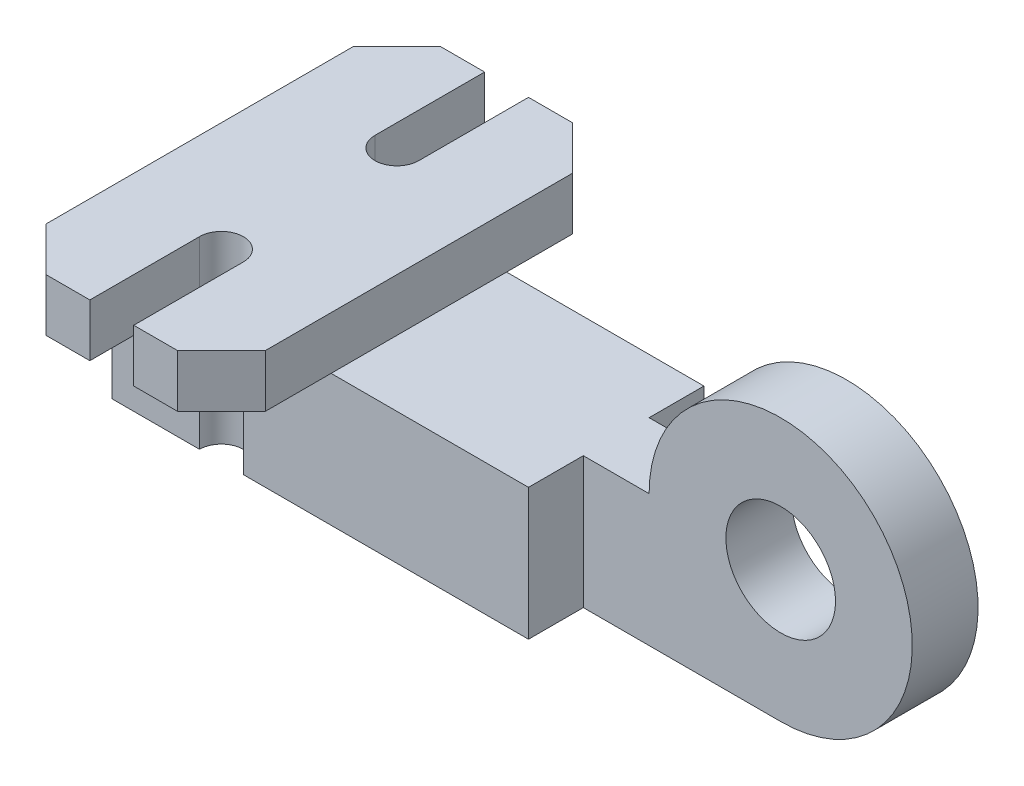
ISO-10303-21;
HEADER;
FILE_DESCRIPTION(('STEP AP214'),'2;1');
FILE_NAME('part.step','',(''),(''),'','','');
FILE_SCHEMA(('AUTOMOTIVE_DESIGN { 1 0 10303 214 1 1 1 1 }'));
ENDSEC;
DATA;
#1=APPLICATION_CONTEXT('core data for automotive mechanical design processes');
#2=APPLICATION_PROTOCOL_DEFINITION('international standard','automotive_design',2000,#1);
#3=PRODUCT_CONTEXT('',#1,'mechanical');
#4=PRODUCT('Part','Part','',(#3));
#5=PRODUCT_RELATED_PRODUCT_CATEGORY('part','',(#4));
#6=PRODUCT_DEFINITION_FORMATION('','',#4);
#7=PRODUCT_DEFINITION_CONTEXT('part definition',#1,'design');
#8=PRODUCT_DEFINITION('design','',#6,#7);
#9=PRODUCT_DEFINITION_SHAPE('','',#8);
#10=(LENGTH_UNIT() NAMED_UNIT(*) SI_UNIT(.MILLI.,.METRE.));
#11=(NAMED_UNIT(*) PLANE_ANGLE_UNIT() SI_UNIT($,.RADIAN.));
#12=(NAMED_UNIT(*) SI_UNIT($,.STERADIAN.) SOLID_ANGLE_UNIT());
#13=UNCERTAINTY_MEASURE_WITH_UNIT(LENGTH_MEASURE(1.E-05),#10,'distance_accuracy_value','');
#14=(GEOMETRIC_REPRESENTATION_CONTEXT(3) GLOBAL_UNCERTAINTY_ASSIGNED_CONTEXT((#13)) GLOBAL_UNIT_ASSIGNED_CONTEXT((#10,
#11,#12)) REPRESENTATION_CONTEXT('',''));
#15=CARTESIAN_POINT('',(0.,0.,0.));
#16=DIRECTION('',(0.,0.,1.));
#17=DIRECTION('',(1.,0.,0.));
#18=AXIS2_PLACEMENT_3D('',#15,#16,#17);
#19=CARTESIAN_POINT('',(0.,0.,20.));
#20=DIRECTION('',(0.,0.,-1.));
#21=DIRECTION('',(-1.,0.,0.));
#22=AXIS2_PLACEMENT_3D('',#19,#20,#21);
#23=PLANE('',#22);
#24=DIRECTION('',(-1.,0.,0.));
#25=VECTOR('',#24,1.);
#26=CARTESIAN_POINT('',(-47.5,15.,20.));
#27=LINE('',#26,#25);
#28=CARTESIAN_POINT('',(2.5,15.,20.));
#29=VERTEX_POINT('',#28);
#30=CARTESIAN_POINT('',(-17.5,15.,20.));
#31=VERTEX_POINT('',#30);
#32=EDGE_CURVE('E343',#29,#31,#27,.T.);
#33=ORIENTED_EDGE('',*,*,#32,.T.);
#34=DIRECTION('',(0.,1.,0.));
#35=VECTOR('',#34,1.);
#36=CARTESIAN_POINT('',(-17.5,-15.,20.));
#37=LINE('',#36,#35);
#38=CARTESIAN_POINT('',(-17.5,-15.,20.));
#39=VERTEX_POINT('',#38);
#40=EDGE_CURVE('E783',#39,#31,#37,.T.);
#41=ORIENTED_EDGE('',*,*,#40,.F.);
#42=DIRECTION('',(1.,0.,0.));
#43=VECTOR('',#42,1.);
#44=CARTESIAN_POINT('',(-47.5,-15.,20.));
#45=LINE('',#44,#43);
#46=CARTESIAN_POINT('',(47.5,-15.,20.));
#47=VERTEX_POINT('',#46);
#48=EDGE_CURVE('E347',#39,#47,#45,.T.);
#49=ORIENTED_EDGE('',*,*,#48,.T.);
#50=DIRECTION('',(0.,1.,0.));
#51=VECTOR('',#50,1.);
#52=CARTESIAN_POINT('',(47.5,-15.,20.));
#53=LINE('',#52,#51);
#54=CARTESIAN_POINT('',(47.5,15.,20.));
#55=VERTEX_POINT('',#54);
#56=EDGE_CURVE('E259',#47,#55,#53,.T.);
#57=ORIENTED_EDGE('',*,*,#56,.T.);
#58=EDGE_CURVE('E337',#55,#29,#27,.T.);
#59=ORIENTED_EDGE('',*,*,#58,.T.);
#60=EDGE_LOOP('',(#33,#41,#49,#57,#59));
#61=FACE_BOUND('',#60,.T.);
#62=ADVANCED_FACE('F50',(#61),#23,.F.);
#63=CARTESIAN_POINT('',(0.,0.,-20.));
#64=DIRECTION('',(0.,0.,-1.));
#65=DIRECTION('',(-1.,0.,0.));
#66=AXIS2_PLACEMENT_3D('',#63,#64,#65);
#67=PLANE('',#66);
#68=DIRECTION('',(0.,1.,0.));
#69=VECTOR('',#68,1.);
#70=CARTESIAN_POINT('',(-27.5,-15.,-20.));
#71=LINE('',#70,#69);
#72=CARTESIAN_POINT('',(-27.5,-15.,-20.));
#73=VERTEX_POINT('',#72);
#74=CARTESIAN_POINT('',(-27.5,15.,-20.));
#75=VERTEX_POINT('',#74);
#76=EDGE_CURVE('E792',#73,#75,#71,.T.);
#77=ORIENTED_EDGE('',*,*,#76,.F.);
#78=DIRECTION('',(1.,0.,0.));
#79=VECTOR('',#78,1.);
#80=CARTESIAN_POINT('',(-47.5,-15.,-20.));
#81=LINE('',#80,#79);
#82=CARTESIAN_POINT('',(-47.5,-15.,-20.));
#83=VERTEX_POINT('',#82);
#84=EDGE_CURVE('E248',#83,#73,#81,.T.);
#85=ORIENTED_EDGE('',*,*,#84,.F.);
#86=DIRECTION('',(0.,-1.,0.));
#87=VECTOR('',#86,1.);
#88=CARTESIAN_POINT('',(-47.5,-15.,-20.));
#89=LINE('',#88,#87);
#90=CARTESIAN_POINT('',(-47.5,15.,-20.));
#91=VERTEX_POINT('',#90);
#92=EDGE_CURVE('E260',#91,#83,#89,.T.);
#93=ORIENTED_EDGE('',*,*,#92,.F.);
#94=DIRECTION('',(-1.,0.,0.));
#95=VECTOR('',#94,1.);
#96=CARTESIAN_POINT('',(-47.5,15.,-20.));
#97=LINE('',#96,#95);
#98=EDGE_CURVE('E348',#75,#91,#97,.T.);
#99=ORIENTED_EDGE('',*,*,#98,.F.);
#100=EDGE_LOOP('',(#77,#85,#93,#99));
#101=FACE_BOUND('',#100,.T.);
#102=ADVANCED_FACE('F364',(#101),#67,.T.);
#103=CARTESIAN_POINT('',(0.,15.,0.));
#104=DIRECTION('',(0.,1.,0.));
#105=DIRECTION('',(0.,0.,1.));
#106=AXIS2_PLACEMENT_3D('',#103,#104,#105);
#107=PLANE('',#106);
#108=DIRECTION('',(0.,0.,1.));
#109=VECTOR('',#108,1.);
#110=CARTESIAN_POINT('',(-47.5,15.,-45.));
#111=LINE('',#110,#109);
#112=CARTESIAN_POINT('',(-47.5,15.,-35.));
#113=VERTEX_POINT('',#112);
#114=EDGE_CURVE('E328',#113,#91,#111,.T.);
#115=ORIENTED_EDGE('',*,*,#114,.F.);
#116=DIRECTION('',(-0.707106781186548,0.,0.707106781186547));
#117=VECTOR('',#116,1.);
#118=CARTESIAN_POINT('',(-47.5,15.,-35.));
#119=LINE('',#118,#117);
#120=CARTESIAN_POINT('',(-37.5,15.,-45.));
#121=VERTEX_POINT('',#120);
#122=EDGE_CURVE('E305',#113,#121,#119,.F.);
#123=ORIENTED_EDGE('',*,*,#122,.T.);
#124=DIRECTION('',(-1.,0.,0.));
#125=VECTOR('',#124,1.);
#126=CARTESIAN_POINT('',(-47.5,15.,-45.));
#127=LINE('',#126,#125);
#128=CARTESIAN_POINT('',(-27.5,15.,-45.));
#129=VERTEX_POINT('',#128);
#130=EDGE_CURVE('E334',#129,#121,#127,.T.);
#131=ORIENTED_EDGE('',*,*,#130,.F.);
#132=DIRECTION('',(0.,0.,1.));
#133=VECTOR('',#132,1.);
#134=CARTESIAN_POINT('',(-27.5,15.,0.));
#135=LINE('',#134,#133);
#136=EDGE_CURVE('E361',#129,#75,#135,.T.);
#137=ORIENTED_EDGE('',*,*,#136,.T.);
#138=ORIENTED_EDGE('',*,*,#98,.T.);
#139=EDGE_LOOP('',(#115,#123,#131,#137,#138));
#140=FACE_BOUND('',#139,.T.);
#141=ADVANCED_FACE('F363',(#140),#107,.F.);
#142=CARTESIAN_POINT('',(-47.5,27.,45.));
#143=DIRECTION('',(0.,0.,-1.));
#144=DIRECTION('',(-1.,0.,0.));
#145=AXIS2_PLACEMENT_3D('',#142,#143,#144);
#146=PLANE('',#145);
#147=DIRECTION('',(1.,0.,0.));
#148=VECTOR('',#147,1.);
#149=CARTESIAN_POINT('',(-47.5,15.,45.));
#150=LINE('',#149,#148);
#151=CARTESIAN_POINT('',(-17.5,15.,45.));
#152=VERTEX_POINT('',#151);
#153=CARTESIAN_POINT('',(-7.50000000000003,15.,45.));
#154=VERTEX_POINT('',#153);
#155=EDGE_CURVE('E322',#152,#154,#150,.T.);
#156=ORIENTED_EDGE('',*,*,#155,.T.);
#157=DIRECTION('',(0.,1.,0.));
#158=VECTOR('',#157,1.);
#159=CARTESIAN_POINT('',(-7.50000000000003,27.,45.));
#160=LINE('',#159,#158);
#161=CARTESIAN_POINT('',(-7.50000000000003,27.,45.));
#162=VERTEX_POINT('',#161);
#163=EDGE_CURVE('E306',#154,#162,#160,.T.);
#164=ORIENTED_EDGE('',*,*,#163,.T.);
#165=DIRECTION('',(1.,0.,0.));
#166=VECTOR('',#165,1.);
#167=CARTESIAN_POINT('',(-47.5,27.,45.));
#168=LINE('',#167,#166);
#169=CARTESIAN_POINT('',(-17.5,27.,45.));
#170=VERTEX_POINT('',#169);
#171=EDGE_CURVE('E392',#170,#162,#168,.T.);
#172=ORIENTED_EDGE('',*,*,#171,.F.);
#173=DIRECTION('',(0.,1.,0.));
#174=VECTOR('',#173,1.);
#175=CARTESIAN_POINT('',(-17.5,-15.,45.));
#176=LINE('',#175,#174);
#177=EDGE_CURVE('E789',#152,#170,#176,.T.);
#178=ORIENTED_EDGE('',*,*,#177,.F.);
#179=EDGE_LOOP('',(#156,#164,#172,#178));
#180=FACE_BOUND('',#179,.T.);
#181=ADVANCED_FACE('F567',(#180),#146,.F.);
#182=CARTESIAN_POINT('',(-47.5,27.,-45.));
#183=DIRECTION('',(0.,0.,1.));
#184=DIRECTION('',(1.,0.,0.));
#185=AXIS2_PLACEMENT_3D('',#182,#183,#184);
#186=PLANE('',#185);
#187=ORIENTED_EDGE('',*,*,#130,.T.);
#188=DIRECTION('',(0.,1.,0.));
#189=VECTOR('',#188,1.);
#190=CARTESIAN_POINT('',(-37.5,27.,-45.));
#191=LINE('',#190,#189);
#192=CARTESIAN_POINT('',(-37.5,27.,-45.));
#193=VERTEX_POINT('',#192);
#194=EDGE_CURVE('E302',#121,#193,#191,.T.);
#195=ORIENTED_EDGE('',*,*,#194,.T.);
#196=DIRECTION('',(-1.,0.,0.));
#197=VECTOR('',#196,1.);
#198=CARTESIAN_POINT('',(-47.5,27.,-45.));
#199=LINE('',#198,#197);
#200=CARTESIAN_POINT('',(-27.5,27.,-45.));
#201=VERTEX_POINT('',#200);
#202=EDGE_CURVE('E398',#201,#193,#199,.T.);
#203=ORIENTED_EDGE('',*,*,#202,.F.);
#204=DIRECTION('',(0.,1.,0.));
#205=VECTOR('',#204,1.);
#206=CARTESIAN_POINT('',(-27.5,-15.,-45.));
#207=LINE('',#206,#205);
#208=EDGE_CURVE('E770',#129,#201,#207,.T.);
#209=ORIENTED_EDGE('',*,*,#208,.F.);
#210=EDGE_LOOP('',(#187,#195,#203,#209));
#211=FACE_BOUND('',#210,.T.);
#212=ADVANCED_FACE('F579',(#211),#186,.F.);
#213=DIRECTION('',(0.,0.,-1.));
#214=VECTOR('',#213,1.);
#215=CARTESIAN_POINT('',(2.49999999999999,15.,-45.));
#216=LINE('',#215,#214);
#217=CARTESIAN_POINT('',(2.5,15.,35.));
#218=VERTEX_POINT('',#217);
#219=EDGE_CURVE('E330',#218,#29,#216,.T.);
#220=ORIENTED_EDGE('',*,*,#219,.F.);
#221=DIRECTION('',(0.707106781186548,0.,-0.707106781186547));
#222=VECTOR('',#221,1.);
#223=CARTESIAN_POINT('',(2.5,15.,35.));
#224=LINE('',#223,#222);
#225=EDGE_CURVE('E68',#218,#154,#224,.F.);
#226=ORIENTED_EDGE('',*,*,#225,.T.);
#227=ORIENTED_EDGE('',*,*,#155,.F.);
#228=DIRECTION('',(0.,0.,-1.));
#229=VECTOR('',#228,1.);
#230=CARTESIAN_POINT('',(-17.5,15.,0.));
#231=LINE('',#230,#229);
#232=EDGE_CURVE('E280',#152,#31,#231,.T.);
#233=ORIENTED_EDGE('',*,*,#232,.T.);
#234=ORIENTED_EDGE('',*,*,#32,.F.);
#235=EDGE_LOOP('',(#220,#226,#227,#233,#234));
#236=FACE_BOUND('',#235,.T.);
#237=ADVANCED_FACE('F566',(#236),#107,.F.);
#238=CARTESIAN_POINT('',(47.5,-15.,20.));
#239=DIRECTION('',(-1.,0.,0.));
#240=DIRECTION('',(0.,0.,1.));
#241=AXIS2_PLACEMENT_3D('',#238,#239,#240);
#242=PLANE('',#241);
#243=DIRECTION('',(0.,-1.,0.));
#244=VECTOR('',#243,1.);
#245=CARTESIAN_POINT('',(47.5,-15.,7.5));
#246=LINE('',#245,#244);
#247=CARTESIAN_POINT('',(47.5,15.,7.5));
#248=VERTEX_POINT('',#247);
#249=CARTESIAN_POINT('',(47.5,-15.,7.5));
#250=VERTEX_POINT('',#249);
#251=EDGE_CURVE('E810',#248,#250,#246,.T.);
#252=ORIENTED_EDGE('',*,*,#251,.F.);
#253=DIRECTION('',(0.,0.,-1.));
#254=VECTOR('',#253,1.);
#255=CARTESIAN_POINT('',(47.5,15.,20.));
#256=LINE('',#255,#254);
#257=EDGE_CURVE('E269',#55,#248,#256,.T.);
#258=ORIENTED_EDGE('',*,*,#257,.F.);
#259=ORIENTED_EDGE('',*,*,#56,.F.);
#260=DIRECTION('',(0.,0.,-1.));
#261=VECTOR('',#260,1.);
#262=CARTESIAN_POINT('',(47.5,-15.,20.));
#263=LINE('',#262,#261);
#264=EDGE_CURVE('E262',#47,#250,#263,.T.);
#265=ORIENTED_EDGE('',*,*,#264,.T.);
#266=EDGE_LOOP('',(#252,#258,#259,#265));
#267=FACE_BOUND('',#266,.T.);
#268=ADVANCED_FACE('F449',(#267),#242,.F.);
#269=CARTESIAN_POINT('',(-47.5,15.,20.));
#270=DIRECTION('',(0.,-1.,0.));
#271=DIRECTION('',(0.,0.,-1.));
#272=AXIS2_PLACEMENT_3D('',#269,#270,#271);
#273=PLANE('',#272);
#274=CARTESIAN_POINT('',(2.49999999999999,15.,-20.));
#275=VERTEX_POINT('',#274);
#276=EDGE_CURVE('E272',#29,#275,#216,.T.);
#277=ORIENTED_EDGE('',*,*,#276,.F.);
#278=ORIENTED_EDGE('',*,*,#58,.F.);
#279=ORIENTED_EDGE('',*,*,#257,.T.);
#280=DIRECTION('',(-1.,0.,0.));
#281=VECTOR('',#280,1.);
#282=CARTESIAN_POINT('',(47.5,15.,7.5));
#283=LINE('',#282,#281);
#284=CARTESIAN_POINT('',(62.5,15.,7.5));
#285=VERTEX_POINT('',#284);
#286=EDGE_CURVE('E805',#285,#248,#283,.T.);
#287=ORIENTED_EDGE('',*,*,#286,.F.);
#288=DIRECTION('',(0.,0.,-1.));
#289=VECTOR('',#288,1.);
#290=CARTESIAN_POINT('',(62.5,15.,7.5));
#291=LINE('',#290,#289);
#292=CARTESIAN_POINT('',(62.5,15.,-7.5));
#293=VERTEX_POINT('',#292);
#294=EDGE_CURVE('E385',#285,#293,#291,.T.);
#295=ORIENTED_EDGE('',*,*,#294,.T.);
#296=DIRECTION('',(-1.,0.,0.));
#297=VECTOR('',#296,1.);
#298=CARTESIAN_POINT('',(47.5,15.,-7.5));
#299=LINE('',#298,#297);
#300=CARTESIAN_POINT('',(47.5,15.,-7.5));
#301=VERTEX_POINT('',#300);
#302=EDGE_CURVE('E803',#293,#301,#299,.T.);
#303=ORIENTED_EDGE('',*,*,#302,.T.);
#304=CARTESIAN_POINT('',(47.5,15.,-20.));
#305=VERTEX_POINT('',#304);
#306=EDGE_CURVE('E267',#301,#305,#256,.T.);
#307=ORIENTED_EDGE('',*,*,#306,.T.);
#308=EDGE_CURVE('E257',#305,#275,#97,.T.);
#309=ORIENTED_EDGE('',*,*,#308,.T.);
#310=EDGE_LOOP('',(#277,#278,#279,#287,#295,#303,#307,#309));
#311=FACE_BOUND('',#310,.T.);
#312=ADVANCED_FACE('F448',(#311),#273,.F.);
#313=ORIENTED_EDGE('',*,*,#306,.F.);
#314=DIRECTION('',(0.,-1.,0.));
#315=VECTOR('',#314,1.);
#316=CARTESIAN_POINT('',(47.5,-15.,-7.5));
#317=LINE('',#316,#315);
#318=CARTESIAN_POINT('',(47.5,-15.,-7.5));
#319=VERTEX_POINT('',#318);
#320=EDGE_CURVE('E816',#301,#319,#317,.T.);
#321=ORIENTED_EDGE('',*,*,#320,.T.);
#322=CARTESIAN_POINT('',(47.5,-15.,-20.));
#323=VERTEX_POINT('',#322);
#324=EDGE_CURVE('E270',#319,#323,#263,.T.);
#325=ORIENTED_EDGE('',*,*,#324,.T.);
#326=DIRECTION('',(0.,1.,0.));
#327=VECTOR('',#326,1.);
#328=CARTESIAN_POINT('',(47.5,-15.,-20.));
#329=LINE('',#328,#327);
#330=EDGE_CURVE('E258',#323,#305,#329,.T.);
#331=ORIENTED_EDGE('',*,*,#330,.T.);
#332=EDGE_LOOP('',(#313,#321,#325,#331));
#333=FACE_BOUND('',#332,.T.);
#334=ADVANCED_FACE('F444',(#333),#242,.F.);
#335=CARTESIAN_POINT('',(-47.5,-15.,20.));
#336=DIRECTION('',(1.,0.,0.));
#337=DIRECTION('',(0.,0.,-1.));
#338=AXIS2_PLACEMENT_3D('',#335,#336,#337);
#339=PLANE('',#338);
#340=DIRECTION('',(0.,0.,1.));
#341=VECTOR('',#340,1.);
#342=CARTESIAN_POINT('',(-47.5,27.,-45.));
#343=LINE('',#342,#341);
#344=CARTESIAN_POINT('',(-47.5,27.,-35.));
#345=VERTEX_POINT('',#344);
#346=CARTESIAN_POINT('',(-47.5,27.,35.));
#347=VERTEX_POINT('',#346);
#348=EDGE_CURVE('E338',#345,#347,#343,.T.);
#349=ORIENTED_EDGE('',*,*,#348,.F.);
#350=DIRECTION('',(0.,-1.,0.));
#351=VECTOR('',#350,1.);
#352=CARTESIAN_POINT('',(-47.5,-15.,-35.));
#353=LINE('',#352,#351);
#354=EDGE_CURVE('E297',#345,#113,#353,.T.);
#355=ORIENTED_EDGE('',*,*,#354,.T.);
#356=ORIENTED_EDGE('',*,*,#114,.T.);
#357=ORIENTED_EDGE('',*,*,#92,.T.);
#358=DIRECTION('',(0.,0.,-1.));
#359=VECTOR('',#358,1.);
#360=CARTESIAN_POINT('',(-47.5,-15.,20.));
#361=LINE('',#360,#359);
#362=CARTESIAN_POINT('',(-47.5,-15.,20.));
#363=VERTEX_POINT('',#362);
#364=EDGE_CURVE('E266',#363,#83,#361,.T.);
#365=ORIENTED_EDGE('',*,*,#364,.F.);
#366=DIRECTION('',(0.,-1.,0.));
#367=VECTOR('',#366,1.);
#368=CARTESIAN_POINT('',(-47.5,-15.,20.));
#369=LINE('',#368,#367);
#370=CARTESIAN_POINT('',(-47.5,15.,20.));
#371=VERTEX_POINT('',#370);
#372=EDGE_CURVE('E345',#371,#363,#369,.T.);
#373=ORIENTED_EDGE('',*,*,#372,.F.);
#374=CARTESIAN_POINT('',(-47.5,15.,35.));
#375=VERTEX_POINT('',#374);
#376=EDGE_CURVE('E377',#371,#375,#111,.T.);
#377=ORIENTED_EDGE('',*,*,#376,.T.);
#378=DIRECTION('',(0.,1.,0.));
#379=VECTOR('',#378,1.);
#380=CARTESIAN_POINT('',(-47.5,-15.,35.));
#381=LINE('',#380,#379);
#382=EDGE_CURVE('E296',#375,#347,#381,.T.);
#383=ORIENTED_EDGE('',*,*,#382,.T.);
#384=EDGE_LOOP('',(#349,#355,#356,#357,#365,#373,#377,#383));
#385=FACE_BOUND('',#384,.T.);
#386=ADVANCED_FACE('F369',(#385),#339,.F.);
#387=CARTESIAN_POINT('',(-47.5,-15.,20.));
#388=DIRECTION('',(0.,1.,0.));
#389=DIRECTION('',(0.,0.,1.));
#390=AXIS2_PLACEMENT_3D('',#387,#388,#389);
#391=PLANE('',#390);
#392=ORIENTED_EDGE('',*,*,#84,.T.);
#393=CARTESIAN_POINT('',(-22.5,-15.,-20.));
#394=DIRECTION('',(0.,1.,0.));
#395=DIRECTION('',(0.,0.,1.));
#396=AXIS2_PLACEMENT_3D('',#393,#394,#395);
#397=CIRCLE('',#396,5.);
#398=CARTESIAN_POINT('',(-17.5,-15.,-20.));
#399=VERTEX_POINT('',#398);
#400=EDGE_CURVE('E234',#73,#399,#397,.T.);
#401=ORIENTED_EDGE('',*,*,#400,.T.);
#402=EDGE_CURVE('E242',#399,#323,#81,.T.);
#403=ORIENTED_EDGE('',*,*,#402,.T.);
#404=ORIENTED_EDGE('',*,*,#324,.F.);
#405=DIRECTION('',(1.,0.,0.));
#406=VECTOR('',#405,1.);
#407=CARTESIAN_POINT('',(92.5,-15.,-7.5));
#408=LINE('',#407,#406);
#409=CARTESIAN_POINT('',(92.5,-15.,-7.5));
#410=VERTEX_POINT('',#409);
#411=EDGE_CURVE('E818',#319,#410,#408,.T.);
#412=ORIENTED_EDGE('',*,*,#411,.T.);
#413=DIRECTION('',(0.,0.,-1.));
#414=VECTOR('',#413,1.);
#415=CARTESIAN_POINT('',(92.5,-15.,7.5));
#416=LINE('',#415,#414);
#417=CARTESIAN_POINT('',(92.5,-15.,7.5));
#418=VERTEX_POINT('',#417);
#419=EDGE_CURVE('E379',#418,#410,#416,.T.);
#420=ORIENTED_EDGE('',*,*,#419,.F.);
#421=DIRECTION('',(1.,0.,0.));
#422=VECTOR('',#421,1.);
#423=CARTESIAN_POINT('',(92.5,-15.,7.5));
#424=LINE('',#423,#422);
#425=EDGE_CURVE('E811',#250,#418,#424,.T.);
#426=ORIENTED_EDGE('',*,*,#425,.F.);
#427=ORIENTED_EDGE('',*,*,#264,.F.);
#428=ORIENTED_EDGE('',*,*,#48,.F.);
#429=CARTESIAN_POINT('',(-22.5,-15.,20.));
#430=DIRECTION('',(0.,1.,0.));
#431=DIRECTION('',(0.,0.,1.));
#432=AXIS2_PLACEMENT_3D('',#429,#430,#431);
#433=CIRCLE('',#432,5.);
#434=CARTESIAN_POINT('',(-27.5,-15.,20.));
#435=VERTEX_POINT('',#434);
#436=EDGE_CURVE('E372',#39,#435,#433,.T.);
#437=ORIENTED_EDGE('',*,*,#436,.T.);
#438=EDGE_CURVE('E350',#363,#435,#45,.T.);
#439=ORIENTED_EDGE('',*,*,#438,.F.);
#440=ORIENTED_EDGE('',*,*,#364,.T.);
#441=EDGE_LOOP('',(#392,#401,#403,#404,#412,#420,#426,#427,#428,#437,#439,#440));
#442=FACE_BOUND('',#441,.T.);
#443=ADVANCED_FACE('F241',(#442),#391,.F.);
#444=ORIENTED_EDGE('',*,*,#438,.T.);
#445=DIRECTION('',(0.,1.,0.));
#446=VECTOR('',#445,1.);
#447=CARTESIAN_POINT('',(-27.5,-15.,20.));
#448=LINE('',#447,#446);
#449=CARTESIAN_POINT('',(-27.5,15.,20.));
#450=VERTEX_POINT('',#449);
#451=EDGE_CURVE('E378',#435,#450,#448,.T.);
#452=ORIENTED_EDGE('',*,*,#451,.T.);
#453=EDGE_CURVE('E339',#450,#371,#27,.T.);
#454=ORIENTED_EDGE('',*,*,#453,.T.);
#455=ORIENTED_EDGE('',*,*,#372,.T.);
#456=EDGE_LOOP('',(#444,#452,#454,#455));
#457=FACE_BOUND('',#456,.T.);
#458=ADVANCED_FACE('F380',(#457),#23,.F.);
#459=DIRECTION('',(0.,1.,0.));
#460=VECTOR('',#459,1.);
#461=CARTESIAN_POINT('',(-17.5,-15.,-20.));
#462=LINE('',#461,#460);
#463=CARTESIAN_POINT('',(-17.5,15.,-20.));
#464=VERTEX_POINT('',#463);
#465=EDGE_CURVE('E230',#399,#464,#462,.T.);
#466=ORIENTED_EDGE('',*,*,#465,.T.);
#467=EDGE_CURVE('E355',#275,#464,#97,.T.);
#468=ORIENTED_EDGE('',*,*,#467,.F.);
#469=ORIENTED_EDGE('',*,*,#308,.F.);
#470=ORIENTED_EDGE('',*,*,#330,.F.);
#471=ORIENTED_EDGE('',*,*,#402,.F.);
#472=EDGE_LOOP('',(#466,#468,#469,#470,#471));
#473=FACE_BOUND('',#472,.T.);
#474=ADVANCED_FACE('F251',(#473),#67,.T.);
#475=CARTESIAN_POINT('',(-7.49999999999999,15.,-45.));
#476=VERTEX_POINT('',#475);
#477=CARTESIAN_POINT('',(-17.5,15.,-45.));
#478=VERTEX_POINT('',#477);
#479=EDGE_CURVE('E331',#476,#478,#127,.T.);
#480=ORIENTED_EDGE('',*,*,#479,.F.);
#481=DIRECTION('',(-0.707106781186547,0.,-0.707106781186549));
#482=VECTOR('',#481,1.);
#483=CARTESIAN_POINT('',(-7.49999999999999,15.,-45.));
#484=LINE('',#483,#482);
#485=CARTESIAN_POINT('',(2.49999999999999,15.,-35.));
#486=VERTEX_POINT('',#485);
#487=EDGE_CURVE('E281',#476,#486,#484,.F.);
#488=ORIENTED_EDGE('',*,*,#487,.T.);
#489=EDGE_CURVE('E323',#275,#486,#216,.T.);
#490=ORIENTED_EDGE('',*,*,#489,.F.);
#491=ORIENTED_EDGE('',*,*,#467,.T.);
#492=DIRECTION('',(0.,0.,-1.));
#493=VECTOR('',#492,1.);
#494=CARTESIAN_POINT('',(-17.5,15.,0.));
#495=LINE('',#494,#493);
#496=EDGE_CURVE('E765',#464,#478,#495,.T.);
#497=ORIENTED_EDGE('',*,*,#496,.T.);
#498=EDGE_LOOP('',(#480,#488,#490,#491,#497));
#499=FACE_BOUND('',#498,.T.);
#500=ADVANCED_FACE('F437',(#499),#107,.F.);
#501=CARTESIAN_POINT('',(-37.5,27.,45.));
#502=VERTEX_POINT('',#501);
#503=CARTESIAN_POINT('',(-27.5,27.,45.));
#504=VERTEX_POINT('',#503);
#505=EDGE_CURVE('E316',#502,#504,#168,.T.);
#506=ORIENTED_EDGE('',*,*,#505,.F.);
#507=DIRECTION('',(0.,-1.,0.));
#508=VECTOR('',#507,1.);
#509=CARTESIAN_POINT('',(-37.5,27.,45.));
#510=LINE('',#509,#508);
#511=CARTESIAN_POINT('',(-37.5,15.,45.));
#512=VERTEX_POINT('',#511);
#513=EDGE_CURVE('E57',#502,#512,#510,.T.);
#514=ORIENTED_EDGE('',*,*,#513,.T.);
#515=CARTESIAN_POINT('',(-27.5,15.,45.));
#516=VERTEX_POINT('',#515);
#517=EDGE_CURVE('E314',#512,#516,#150,.T.);
#518=ORIENTED_EDGE('',*,*,#517,.T.);
#519=DIRECTION('',(0.,1.,0.));
#520=VECTOR('',#519,1.);
#521=CARTESIAN_POINT('',(-27.5,-15.,45.));
#522=LINE('',#521,#520);
#523=EDGE_CURVE('E793',#516,#504,#522,.T.);
#524=ORIENTED_EDGE('',*,*,#523,.T.);
#525=EDGE_LOOP('',(#506,#514,#518,#524));
#526=FACE_BOUND('',#525,.T.);
#527=ADVANCED_FACE('F315',(#526),#146,.F.);
#528=CARTESIAN_POINT('',(2.49999999999999,27.,-45.));
#529=DIRECTION('',(-1.,0.,0.));
#530=DIRECTION('',(0.,0.,1.));
#531=AXIS2_PLACEMENT_3D('',#528,#529,#530);
#532=PLANE('',#531);
#533=ORIENTED_EDGE('',*,*,#489,.T.);
#534=DIRECTION('',(0.,1.,0.));
#535=VECTOR('',#534,1.);
#536=CARTESIAN_POINT('',(2.49999999999999,27.,-35.));
#537=LINE('',#536,#535);
#538=CARTESIAN_POINT('',(2.49999999999999,27.,-35.));
#539=VERTEX_POINT('',#538);
#540=EDGE_CURVE('E290',#486,#539,#537,.T.);
#541=ORIENTED_EDGE('',*,*,#540,.T.);
#542=DIRECTION('',(0.,0.,-1.));
#543=VECTOR('',#542,1.);
#544=CARTESIAN_POINT('',(2.49999999999999,27.,-45.));
#545=LINE('',#544,#543);
#546=CARTESIAN_POINT('',(2.5,27.,35.));
#547=VERTEX_POINT('',#546);
#548=EDGE_CURVE('E396',#547,#539,#545,.T.);
#549=ORIENTED_EDGE('',*,*,#548,.F.);
#550=DIRECTION('',(0.,-1.,0.));
#551=VECTOR('',#550,1.);
#552=CARTESIAN_POINT('',(2.5,27.,35.));
#553=LINE('',#552,#551);
#554=EDGE_CURVE('E282',#547,#218,#553,.T.);
#555=ORIENTED_EDGE('',*,*,#554,.T.);
#556=ORIENTED_EDGE('',*,*,#219,.T.);
#557=ORIENTED_EDGE('',*,*,#276,.T.);
#558=EDGE_LOOP('',(#533,#541,#549,#555,#556,#557));
#559=FACE_BOUND('',#558,.T.);
#560=ADVANCED_FACE('F656',(#559),#532,.F.);
#561=CARTESIAN_POINT('',(-7.49999999999999,27.,-45.));
#562=VERTEX_POINT('',#561);
#563=CARTESIAN_POINT('',(-17.5,27.,-45.));
#564=VERTEX_POINT('',#563);
#565=EDGE_CURVE('E353',#562,#564,#199,.T.);
#566=ORIENTED_EDGE('',*,*,#565,.F.);
#567=DIRECTION('',(0.,-1.,0.));
#568=VECTOR('',#567,1.);
#569=CARTESIAN_POINT('',(-7.49999999999999,27.,-45.));
#570=LINE('',#569,#568);
#571=EDGE_CURVE('E278',#562,#476,#570,.T.);
#572=ORIENTED_EDGE('',*,*,#571,.T.);
#573=ORIENTED_EDGE('',*,*,#479,.T.);
#574=DIRECTION('',(0.,1.,0.));
#575=VECTOR('',#574,1.);
#576=CARTESIAN_POINT('',(-17.5,-15.,-45.));
#577=LINE('',#576,#575);
#578=EDGE_CURVE('E239',#478,#564,#577,.T.);
#579=ORIENTED_EDGE('',*,*,#578,.T.);
#580=EDGE_LOOP('',(#566,#572,#573,#579));
#581=FACE_BOUND('',#580,.T.);
#582=ADVANCED_FACE('F588',(#581),#186,.F.);
#583=CARTESIAN_POINT('',(0.,27.,0.));
#584=DIRECTION('',(0.,1.,0.));
#585=DIRECTION('',(0.,0.,1.));
#586=AXIS2_PLACEMENT_3D('',#583,#584,#585);
#587=PLANE('',#586);
#588=ORIENTED_EDGE('',*,*,#548,.T.);
#589=DIRECTION('',(0.707106781186547,0.,0.707106781186549));
#590=VECTOR('',#589,1.);
#591=CARTESIAN_POINT('',(18.75,27.,-18.75));
#592=LINE('',#591,#590);
#593=EDGE_CURVE('E298',#539,#562,#592,.F.);
#594=ORIENTED_EDGE('',*,*,#593,.T.);
#595=ORIENTED_EDGE('',*,*,#565,.T.);
#596=DIRECTION('',(0.,0.,-1.));
#597=VECTOR('',#596,1.);
#598=CARTESIAN_POINT('',(-17.5,27.,-45.));
#599=LINE('',#598,#597);
#600=CARTESIAN_POINT('',(-17.5,27.,-20.));
#601=VERTEX_POINT('',#600);
#602=EDGE_CURVE('E766',#601,#564,#599,.T.);
#603=ORIENTED_EDGE('',*,*,#602,.F.);
#604=CARTESIAN_POINT('',(-22.5,27.,-20.));
#605=DIRECTION('',(0.,1.,0.));
#606=DIRECTION('',(0.,0.,1.));
#607=AXIS2_PLACEMENT_3D('',#604,#605,#606);
#608=CIRCLE('',#607,5.);
#609=CARTESIAN_POINT('',(-27.5,27.,-20.));
#610=VERTEX_POINT('',#609);
#611=EDGE_CURVE('E790',#610,#601,#608,.T.);
#612=ORIENTED_EDGE('',*,*,#611,.F.);
#613=DIRECTION('',(0.,0.,1.));
#614=VECTOR('',#613,1.);
#615=CARTESIAN_POINT('',(-27.5,27.,-20.));
#616=LINE('',#615,#614);
#617=EDGE_CURVE('E247',#201,#610,#616,.T.);
#618=ORIENTED_EDGE('',*,*,#617,.F.);
#619=ORIENTED_EDGE('',*,*,#202,.T.);
#620=DIRECTION('',(0.707106781186548,0.,-0.707106781186547));
#621=VECTOR('',#620,1.);
#622=CARTESIAN_POINT('',(-41.2499999999999,27.,-41.25));
#623=LINE('',#622,#621);
#624=EDGE_CURVE('E294',#193,#345,#623,.F.);
#625=ORIENTED_EDGE('',*,*,#624,.T.);
#626=ORIENTED_EDGE('',*,*,#348,.T.);
#627=DIRECTION('',(-0.707106781186547,0.,-0.707106781186549));
#628=VECTOR('',#627,1.);
#629=CARTESIAN_POINT('',(-41.2500000000001,27.,41.2499999999999));
#630=LINE('',#629,#628);
#631=EDGE_CURVE('E287',#347,#502,#630,.F.);
#632=ORIENTED_EDGE('',*,*,#631,.T.);
#633=ORIENTED_EDGE('',*,*,#505,.T.);
#634=DIRECTION('',(0.,0.,1.));
#635=VECTOR('',#634,1.);
#636=CARTESIAN_POINT('',(-27.5,27.,20.));
#637=LINE('',#636,#635);
#638=CARTESIAN_POINT('',(-27.5,27.,20.));
#639=VERTEX_POINT('',#638);
#640=EDGE_CURVE('E779',#639,#504,#637,.T.);
#641=ORIENTED_EDGE('',*,*,#640,.F.);
#642=CARTESIAN_POINT('',(-22.5,27.,20.));
#643=DIRECTION('',(0.,1.,0.));
#644=DIRECTION('',(0.,0.,1.));
#645=AXIS2_PLACEMENT_3D('',#642,#643,#644);
#646=CIRCLE('',#645,5.);
#647=CARTESIAN_POINT('',(-17.5,27.,20.));
#648=VERTEX_POINT('',#647);
#649=EDGE_CURVE('E778',#648,#639,#646,.T.);
#650=ORIENTED_EDGE('',*,*,#649,.F.);
#651=DIRECTION('',(0.,0.,-1.));
#652=VECTOR('',#651,1.);
#653=CARTESIAN_POINT('',(-17.5,27.,45.));
#654=LINE('',#653,#652);
#655=EDGE_CURVE('E773',#170,#648,#654,.T.);
#656=ORIENTED_EDGE('',*,*,#655,.F.);
#657=ORIENTED_EDGE('',*,*,#171,.T.);
#658=DIRECTION('',(-0.707106781186548,0.,0.707106781186547));
#659=VECTOR('',#658,1.);
#660=CARTESIAN_POINT('',(18.75,27.,18.75));
#661=LINE('',#660,#659);
#662=EDGE_CURVE('E295',#162,#547,#661,.F.);
#663=ORIENTED_EDGE('',*,*,#662,.T.);
#664=EDGE_LOOP('',(#588,#594,#595,#603,#612,#618,#619,#625,#626,#632,#633,#641,#650,#656,#657,#663));
#665=FACE_BOUND('',#664,.T.);
#666=ADVANCED_FACE('F406',(#665),#587,.T.);
#667=ORIENTED_EDGE('',*,*,#517,.F.);
#668=DIRECTION('',(0.707106781186547,0.,0.707106781186549));
#669=VECTOR('',#668,1.);
#670=CARTESIAN_POINT('',(-37.5,15.,45.));
#671=LINE('',#670,#669);
#672=EDGE_CURVE('E11',#512,#375,#671,.F.);
#673=ORIENTED_EDGE('',*,*,#672,.T.);
#674=ORIENTED_EDGE('',*,*,#376,.F.);
#675=ORIENTED_EDGE('',*,*,#453,.F.);
#676=DIRECTION('',(0.,0.,1.));
#677=VECTOR('',#676,1.);
#678=CARTESIAN_POINT('',(-27.5,15.,0.));
#679=LINE('',#678,#677);
#680=EDGE_CURVE('E273',#450,#516,#679,.T.);
#681=ORIENTED_EDGE('',*,*,#680,.T.);
#682=EDGE_LOOP('',(#667,#673,#674,#675,#681));
#683=FACE_BOUND('',#682,.T.);
#684=ADVANCED_FACE('F317',(#683),#107,.F.);
#685=CARTESIAN_POINT('',(92.5,15.,7.5));
#686=DIRECTION('',(0.,0.,-1.));
#687=DIRECTION('',(-1.,0.,0.));
#688=AXIS2_PLACEMENT_3D('',#685,#686,#687);
#689=CYLINDRICAL_SURFACE('',#688,30.);
#690=CARTESIAN_POINT('',(92.5,15.,-7.5));
#691=DIRECTION('',(0.,0.,1.));
#692=DIRECTION('',(1.,0.,0.));
#693=AXIS2_PLACEMENT_3D('',#690,#691,#692);
#694=CIRCLE('',#693,30.);
#695=EDGE_CURVE('E806',#410,#293,#694,.T.);
#696=ORIENTED_EDGE('',*,*,#695,.T.);
#697=ORIENTED_EDGE('',*,*,#294,.F.);
#698=CARTESIAN_POINT('',(92.5,15.,7.5));
#699=DIRECTION('',(0.,0.,1.));
#700=DIRECTION('',(1.,0.,0.));
#701=AXIS2_PLACEMENT_3D('',#698,#699,#700);
#702=CIRCLE('',#701,30.);
#703=EDGE_CURVE('E386',#418,#285,#702,.T.);
#704=ORIENTED_EDGE('',*,*,#703,.F.);
#705=ORIENTED_EDGE('',*,*,#419,.T.);
#706=EDGE_LOOP('',(#696,#697,#704,#705));
#707=FACE_BOUND('',#706,.T.);
#708=ADVANCED_FACE('F618',(#707),#689,.T.);
#709=CARTESIAN_POINT('',(92.5,15.,7.5));
#710=DIRECTION('',(0.,0.,1.));
#711=DIRECTION('',(1.,0.,0.));
#712=AXIS2_PLACEMENT_3D('',#709,#710,#711);
#713=PLANE('',#712);
#714=CARTESIAN_POINT('',(92.5,15.,7.5));
#715=DIRECTION('',(0.,0.,1.));
#716=DIRECTION('',(1.,0.,0.));
#717=AXIS2_PLACEMENT_3D('',#714,#715,#716);
#718=CIRCLE('',#717,12.5);
#719=CARTESIAN_POINT('',(105.,15.,7.5));
#720=VERTEX_POINT('',#719);
#721=EDGE_CURVE('E796',#720,#720,#718,.T.);
#722=ORIENTED_EDGE('',*,*,#721,.F.);
#723=EDGE_LOOP('',(#722));
#724=FACE_BOUND('',#723,.T.);
#725=ORIENTED_EDGE('',*,*,#286,.T.);
#726=ORIENTED_EDGE('',*,*,#251,.T.);
#727=ORIENTED_EDGE('',*,*,#425,.T.);
#728=ORIENTED_EDGE('',*,*,#703,.T.);
#729=EDGE_LOOP('',(#725,#726,#727,#728));
#730=FACE_BOUND('',#729,.T.);
#731=ADVANCED_FACE('F608',(#724,#730),#713,.T.);
#732=CARTESIAN_POINT('',(92.5,15.,-7.5));
#733=DIRECTION('',(0.,0.,1.));
#734=DIRECTION('',(1.,0.,0.));
#735=AXIS2_PLACEMENT_3D('',#732,#733,#734);
#736=PLANE('',#735);
#737=CARTESIAN_POINT('',(92.5,15.,-7.5));
#738=DIRECTION('',(0.,0.,1.));
#739=DIRECTION('',(1.,0.,0.));
#740=AXIS2_PLACEMENT_3D('',#737,#738,#739);
#741=CIRCLE('',#740,12.5);
#742=CARTESIAN_POINT('',(105.,15.,-7.5));
#743=VERTEX_POINT('',#742);
#744=EDGE_CURVE('E800',#743,#743,#741,.T.);
#745=ORIENTED_EDGE('',*,*,#744,.T.);
#746=EDGE_LOOP('',(#745));
#747=FACE_BOUND('',#746,.T.);
#748=ORIENTED_EDGE('',*,*,#302,.F.);
#749=ORIENTED_EDGE('',*,*,#695,.F.);
#750=ORIENTED_EDGE('',*,*,#411,.F.);
#751=ORIENTED_EDGE('',*,*,#320,.F.);
#752=EDGE_LOOP('',(#748,#749,#750,#751));
#753=FACE_BOUND('',#752,.T.);
#754=ADVANCED_FACE('F601',(#747,#753),#736,.F.);
#755=CARTESIAN_POINT('',(92.5,15.,-7.5));
#756=DIRECTION('',(0.,0.,1.));
#757=DIRECTION('',(1.,0.,0.));
#758=AXIS2_PLACEMENT_3D('',#755,#756,#757);
#759=CYLINDRICAL_SURFACE('',#758,12.5);
#760=ORIENTED_EDGE('',*,*,#744,.F.);
#761=EDGE_LOOP('',(#760));
#762=FACE_BOUND('',#761,.T.);
#763=ORIENTED_EDGE('',*,*,#721,.T.);
#764=EDGE_LOOP('',(#763));
#765=FACE_BOUND('',#764,.T.);
#766=ADVANCED_FACE('F544',(#762,#765),#759,.F.);
#767=CARTESIAN_POINT('',(-17.5,-15.,45.));
#768=DIRECTION('',(1.,0.,0.));
#769=DIRECTION('',(0.,0.,-1.));
#770=AXIS2_PLACEMENT_3D('',#767,#768,#769);
#771=PLANE('',#770);
#772=ORIENTED_EDGE('',*,*,#177,.T.);
#773=ORIENTED_EDGE('',*,*,#655,.T.);
#774=EDGE_CURVE('E786',#31,#648,#37,.T.);
#775=ORIENTED_EDGE('',*,*,#774,.F.);
#776=ORIENTED_EDGE('',*,*,#232,.F.);
#777=EDGE_LOOP('',(#772,#773,#775,#776));
#778=FACE_BOUND('',#777,.T.);
#779=ADVANCED_FACE('F536',(#778),#771,.F.);
#780=CARTESIAN_POINT('',(-27.5,-15.,20.));
#781=DIRECTION('',(-1.,0.,0.));
#782=DIRECTION('',(0.,0.,1.));
#783=AXIS2_PLACEMENT_3D('',#780,#781,#782);
#784=PLANE('',#783);
#785=EDGE_CURVE('E771',#450,#639,#448,.T.);
#786=ORIENTED_EDGE('',*,*,#785,.T.);
#787=ORIENTED_EDGE('',*,*,#640,.T.);
#788=ORIENTED_EDGE('',*,*,#523,.F.);
#789=ORIENTED_EDGE('',*,*,#680,.F.);
#790=EDGE_LOOP('',(#786,#787,#788,#789));
#791=FACE_BOUND('',#790,.T.);
#792=ADVANCED_FACE('F528',(#791),#784,.F.);
#793=CARTESIAN_POINT('',(-22.5,-15.,20.));
#794=DIRECTION('',(0.,1.,0.));
#795=DIRECTION('',(0.,0.,1.));
#796=AXIS2_PLACEMENT_3D('',#793,#794,#795);
#797=CYLINDRICAL_SURFACE('',#796,5.);
#798=ORIENTED_EDGE('',*,*,#649,.T.);
#799=ORIENTED_EDGE('',*,*,#785,.F.);
#800=ORIENTED_EDGE('',*,*,#451,.F.);
#801=ORIENTED_EDGE('',*,*,#436,.F.);
#802=ORIENTED_EDGE('',*,*,#40,.T.);
#803=ORIENTED_EDGE('',*,*,#774,.T.);
#804=EDGE_LOOP('',(#798,#799,#800,#801,#802,#803));
#805=FACE_BOUND('',#804,.T.);
#806=ADVANCED_FACE('F518',(#805),#797,.F.);
#807=CARTESIAN_POINT('',(-27.5,-15.,-20.));
#808=DIRECTION('',(-1.,0.,0.));
#809=DIRECTION('',(0.,0.,1.));
#810=AXIS2_PLACEMENT_3D('',#807,#808,#809);
#811=PLANE('',#810);
#812=ORIENTED_EDGE('',*,*,#208,.T.);
#813=ORIENTED_EDGE('',*,*,#617,.T.);
#814=EDGE_CURVE('E768',#75,#610,#71,.T.);
#815=ORIENTED_EDGE('',*,*,#814,.F.);
#816=ORIENTED_EDGE('',*,*,#136,.F.);
#817=EDGE_LOOP('',(#812,#813,#815,#816));
#818=FACE_BOUND('',#817,.T.);
#819=ADVANCED_FACE('F509',(#818),#811,.F.);
#820=CARTESIAN_POINT('',(-17.5,-15.,-45.));
#821=DIRECTION('',(1.,0.,0.));
#822=DIRECTION('',(0.,0.,-1.));
#823=AXIS2_PLACEMENT_3D('',#820,#821,#822);
#824=PLANE('',#823);
#825=EDGE_CURVE('E233',#464,#601,#462,.T.);
#826=ORIENTED_EDGE('',*,*,#825,.T.);
#827=ORIENTED_EDGE('',*,*,#602,.T.);
#828=ORIENTED_EDGE('',*,*,#578,.F.);
#829=ORIENTED_EDGE('',*,*,#496,.F.);
#830=EDGE_LOOP('',(#826,#827,#828,#829));
#831=FACE_BOUND('',#830,.T.);
#832=ADVANCED_FACE('F500',(#831),#824,.F.);
#833=CARTESIAN_POINT('',(-22.5,-15.,-20.));
#834=DIRECTION('',(0.,1.,0.));
#835=DIRECTION('',(0.,0.,1.));
#836=AXIS2_PLACEMENT_3D('',#833,#834,#835);
#837=CYLINDRICAL_SURFACE('',#836,5.);
#838=ORIENTED_EDGE('',*,*,#611,.T.);
#839=ORIENTED_EDGE('',*,*,#825,.F.);
#840=ORIENTED_EDGE('',*,*,#465,.F.);
#841=ORIENTED_EDGE('',*,*,#400,.F.);
#842=ORIENTED_EDGE('',*,*,#76,.T.);
#843=ORIENTED_EDGE('',*,*,#814,.T.);
#844=EDGE_LOOP('',(#838,#839,#840,#841,#842,#843));
#845=FACE_BOUND('',#844,.T.);
#846=ADVANCED_FACE('F229',(#845),#837,.F.);
#847=CARTESIAN_POINT('',(-7.49999999999999,27.,-45.));
#848=DIRECTION('',(-0.707106781186549,0.,0.707106781186547));
#849=DIRECTION('',(0.,-1.,0.));
#850=AXIS2_PLACEMENT_3D('',#847,#848,#849);
#851=PLANE('',#850);
#852=ORIENTED_EDGE('',*,*,#593,.F.);
#853=ORIENTED_EDGE('',*,*,#540,.F.);
#854=ORIENTED_EDGE('',*,*,#487,.F.);
#855=ORIENTED_EDGE('',*,*,#571,.F.);
#856=EDGE_LOOP('',(#852,#853,#854,#855));
#857=FACE_BOUND('',#856,.T.);
#858=ADVANCED_FACE('F453',(#857),#851,.F.);
#859=CARTESIAN_POINT('',(-47.5,-15.,-35.));
#860=DIRECTION('',(0.707106781186547,0.,0.707106781186548));
#861=DIRECTION('',(0.,-1.,0.));
#862=AXIS2_PLACEMENT_3D('',#859,#860,#861);
#863=PLANE('',#862);
#864=ORIENTED_EDGE('',*,*,#624,.F.);
#865=ORIENTED_EDGE('',*,*,#194,.F.);
#866=ORIENTED_EDGE('',*,*,#122,.F.);
#867=ORIENTED_EDGE('',*,*,#354,.F.);
#868=EDGE_LOOP('',(#864,#865,#866,#867));
#869=FACE_BOUND('',#868,.T.);
#870=ADVANCED_FACE('F418',(#869),#863,.F.);
#871=CARTESIAN_POINT('',(2.5,27.,35.));
#872=DIRECTION('',(-0.707106781186547,0.,-0.707106781186548));
#873=DIRECTION('',(0.,-1.,0.));
#874=AXIS2_PLACEMENT_3D('',#871,#872,#873);
#875=PLANE('',#874);
#876=ORIENTED_EDGE('',*,*,#662,.F.);
#877=ORIENTED_EDGE('',*,*,#163,.F.);
#878=ORIENTED_EDGE('',*,*,#225,.F.);
#879=ORIENTED_EDGE('',*,*,#554,.F.);
#880=EDGE_LOOP('',(#876,#877,#878,#879));
#881=FACE_BOUND('',#880,.T.);
#882=ADVANCED_FACE('F416',(#881),#875,.F.);
#883=CARTESIAN_POINT('',(-37.5,27.,45.));
#884=DIRECTION('',(0.707106781186548,0.,-0.707106781186546));
#885=DIRECTION('',(0.,-1.,0.));
#886=AXIS2_PLACEMENT_3D('',#883,#884,#885);
#887=PLANE('',#886);
#888=ORIENTED_EDGE('',*,*,#631,.F.);
#889=ORIENTED_EDGE('',*,*,#382,.F.);
#890=ORIENTED_EDGE('',*,*,#672,.F.);
#891=ORIENTED_EDGE('',*,*,#513,.F.);
#892=EDGE_LOOP('',(#888,#889,#890,#891));
#893=FACE_BOUND('',#892,.T.);
#894=ADVANCED_FACE('F49',(#893),#887,.F.);
#895=CLOSED_SHELL('',(#62,#102,#141,#181,#212,#237,#268,#312,#334,#386,#443,#458,#474,#500,#527,
#560,#582,#666,#684,#708,#731,#754,#766,#779,#792,#806,#819,#832,#846,#858,#870,#882,#894));
#896=MANIFOLD_SOLID_BREP('B2',#895);
#897=ADVANCED_BREP_SHAPE_REPRESENTATION('',(#18,#896),#14);
#898=SHAPE_DEFINITION_REPRESENTATION(#9,#897);
ENDSEC;
END-ISO-10303-21;
